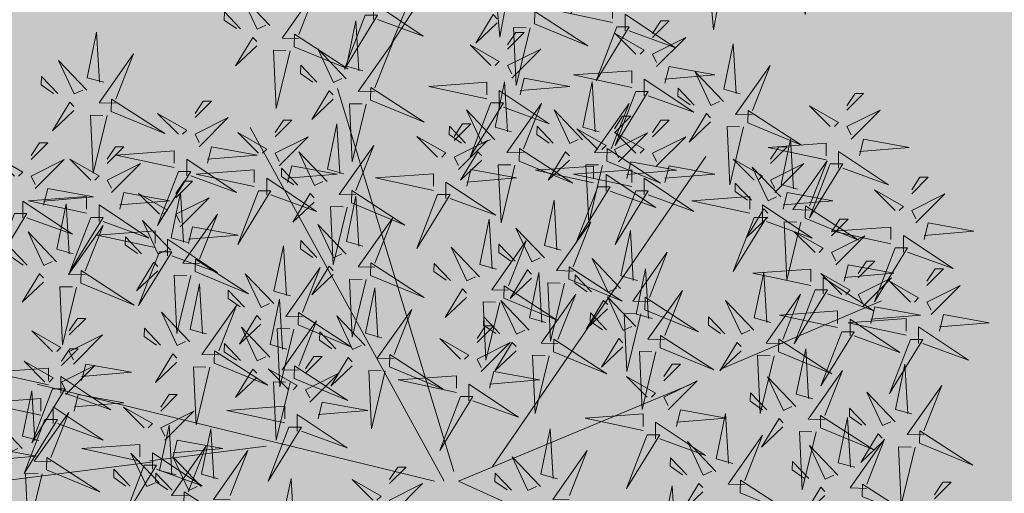
# Model space of a CAD drawing. Units: inches. Extents: x 1704 to 6393, y -157 to 1172.
# Tile 109 of 122: x 2688 to 2716, y 989 to 1003. Entities that reach past the tile are written whole.
import ezdxf

# ---------------------------------------------------------------- set-up
doc = ezdxf.new("R2010")
doc.units = ezdxf.units.IN
doc.header["$MEASUREMENT"] = 0
doc.layers.add('A-ANNO-DIMS', color=7, linetype='Continuous', lineweight=13)
doc.layers.add('L-shrub', color=74, linetype='Continuous', lineweight=18)
doc.layers.add('L-HRDS-PATT', color=9, linetype='Continuous', lineweight=13, true_color=0xc5c1ba)
doc.styles.get("Standard").update_dxf_attribs({"font": 'arial.ttf'})
doc.dimstyles.get("Standard").update_dxf_attribs({"dimtxt": 6, "dimasz": 2, "dimexe": 0.18, "dimexo": 0.0625, "dimgap": 0.09, "dimtad": 0, "dimtih": 1, "dimtoh": 1, "dimdec": 1, "dimzin": 0, "dimdsep": 46, "dimlunit": 3, "dimtxsty": 'Standard', "dimblk": 'ARCHTICK', "dimcen": 0.09, "dimadec": 0, "dimazin": 0, "dimtfac": 1, "dimtdec": 1, "dimtofl": 0, "dimtmove": 0, "dimatfit": 3, "dimfxl": 1, "dimtolj": 1, "dimtzin": 0, "dimarcsym": 0})

# ---------------------------------------------------------------- blocks, each defined once
blk = doc.blocks.new('shrub3')
for p, q in [((-68.47, 143.52), (-106.19, 232.32)), ((-5.99, -2.5), (58.67, 140.12)), ((-14.08, 16.34), (-186.51, 134.74)), ((-5.99, -2.5), (-59.88, 126.66)), ((-11.38, -5.19), (-224.23, -69.78)), ((-5.99, -10.57), (-202.68, -118.21)), ((-5.99, -15.96), (-59.88, -236.62)), ((-17.27, -174.02), (-25.36, -109.43)), ((-16.77, -172.03), (-3.3, -276.98))]:
    blk.add_line(p, q)
for points in [[(29.32, 268.76), (20.08, 271.07), (24.7, 296.43), (27.01, 268.76)], [(72.58, 270.39), (84.86, 300.11), (65.67, 270.57), (72.58, 270.39)], [(-89.4, 264.53), (-98.64, 266.83), (-94.02, 292.2), (-91.71, 264.53)], [(-140.28, 256.06), (-149.52, 258.36), (-144.9, 283.73), (-142.59, 256.06)], [(-82.48, 253), (-91.71, 253), (-73.24, 280.67), (-82.48, 255.31)], [(-27.06, 253.45), (-14.78, 283.17), (-33.97, 253.63), (-27.06, 253.45)], [(-98.64, 259.92), (-114.8, 276.06), (-105.56, 257.61), (-100.94, 259.92)], [(-133.36, 244.53), (-142.59, 244.53), (-124.12, 272.2), (-133.36, 246.84)], [(3.92, 261.85), (-5.31, 271.07), (-5.31, 266.46), (1.62, 261.85)], [(-149.52, 251.45), (-165.68, 267.59), (-156.44, 249.14), (-151.83, 251.45)], [(-114.8, 257.61), (-124.03, 266.83), (-124.03, 262.22), (-117.11, 257.61)], [(-31.61, 255.88), (-31.84, 246.65), (-59.04, 265.8), (-33.91, 255.94)], [(-165.68, 249.14), (-174.91, 258.36), (-174.91, 253.75), (-167.99, 249.14)], [(-105.56, 248.39), (-117.11, 236.86), (-107.87, 253), (-105.56, 250.69)], [(-93.64, 226.42), (-102.88, 228.72), (-98.26, 254.08), (-95.95, 226.42)], [(-84.78, 248.39), (-54.77, 236.86), (-84.78, 255.31), (-84.78, 248.39)], [(-186.92, 220.06), (-196.16, 222.37), (-191.54, 247.73), (-189.23, 220.06)], [(-135.66, 239.92), (-105.65, 228.39), (-135.66, 246.84), (-135.66, 239.92)], [(-43.31, 249.24), (-45.84, 240.07), (-71.08, 245.32), (-43.37, 246.93)], [(-24.81, 251.09), (7.29, 243.36), (-25.04, 241.86), (-24.87, 248.78)], [(2.62, 221.69), (14.9, 251.41), (-4.29, 221.87), (2.62, 221.69)], [(-156.44, 239.92), (-167.99, 228.39), (-158.75, 244.53), (-156.44, 242.22)], [(-87.09, 246.08), (-94.02, 213.8), (-96.33, 246.08), (-89.4, 246.08)], [(-86.72, 214.89), (-95.95, 214.89), (-77.48, 242.56), (-86.72, 217.19)], [(-180, 208.53), (-189.23, 208.53), (-170.76, 236.2), (-180, 210.84)], [(-137.97, 237.61), (-144.9, 205.33), (-147.21, 237.61), (-140.28, 237.61)], [(-116.96, 211.59), (-126.2, 213.9), (-121.58, 239.26), (-119.27, 211.59)], [(-102.88, 221.8), (-119.04, 237.94), (-109.8, 219.5), (-105.18, 221.8)], [(-38.93, 239.9), (-55.47, 224.14), (-36.8, 232.91), (-38.99, 237.59)], [(-196.16, 215.45), (-212.32, 231.59), (-203.08, 213.15), (-198.47, 215.45)], [(-27.58, 232.68), (-16.34, 220.86), (-32.24, 230.49), (-29.88, 232.74)], [(-1.93, 224.12), (-2.16, 214.89), (-29.36, 234.04), (-4.23, 224.17)], [(-119.04, 219.5), (-128.27, 228.72), (-128.27, 224.11), (-121.35, 219.5)], [(-110.04, 200.06), (-119.27, 200.06), (-100.8, 227.73), (-110.04, 202.37)], [(-35.54, 198.4), (-23.26, 228.12), (-42.45, 198.58), (-35.54, 198.4)], [(-212.32, 213.15), (-221.55, 222.37), (-221.55, 217.76), (-214.63, 213.15)], [(-152.14, 189.93), (-139.86, 219.65), (-159.05, 190.11), (-152.14, 189.93)], [(-126.2, 206.98), (-142.36, 223.12), (-133.12, 204.68), (-128.5, 206.98)], [(-37.03, 223.68), (-46.48, 214.68), (-41.87, 214.57), (-37.09, 221.37)], [(-142.36, 204.68), (-151.59, 213.9), (-151.59, 209.29), (-144.67, 204.68)], [(-109.8, 210.27), (-121.35, 198.75), (-112.11, 214.89), (-109.8, 212.58)], [(-89.02, 210.27), (-59.01, 198.75), (-89.02, 217.19), (-89.02, 210.27)], [(-13.63, 217.48), (-16.16, 208.31), (-41.4, 213.56), (-13.69, 215.17)], [(-203.08, 203.92), (-214.63, 192.39), (-205.39, 208.53), (-203.08, 206.23)], [(-182.31, 203.92), (-152.29, 192.39), (-182.31, 210.84), (-182.31, 203.92)], [(-91.33, 207.97), (-98.26, 175.69), (-100.57, 207.97), (-93.64, 207.97)], [(-40.09, 200.83), (-40.32, 191.59), (-67.52, 210.75), (-42.39, 200.88)], [(-9.25, 208.13), (-25.79, 192.38), (-7.12, 201.15), (-9.31, 205.83)], [(-157.24, 177.72), (-166.48, 180.02), (-161.86, 205.38), (-159.55, 177.72)], [(-112.34, 195.45), (-82.33, 183.92), (-112.34, 202.37), (-112.34, 195.45)], [(-77.94, 175.11), (-65.66, 204.83), (-84.85, 175.28), (-77.94, 175.11)], [(-184.61, 201.62), (-191.54, 169.34), (-193.85, 201.62), (-186.92, 201.62)], [(-156.69, 192.36), (-156.92, 183.12), (-184.12, 202.28), (-159, 192.41)], [(-133.12, 195.45), (-144.67, 183.92), (-135.43, 200.06), (-133.12, 197.76)], [(2.1, 200.92), (13.34, 189.09), (-2.56, 198.73), (-0.2, 200.98)], [(-150.32, 166.19), (-159.55, 166.19), (-141.08, 193.86), (-150.32, 168.49)], [(-114.65, 193.15), (-121.58, 160.87), (-123.89, 193.15), (-116.96, 193.15)], [(-51.79, 194.19), (-54.32, 185.02), (-79.56, 190.27), (-51.85, 191.88)], [(-33.29, 196.04), (-1.19, 188.31), (-33.52, 186.81), (-33.35, 193.73)], [(-7.35, 191.92), (-16.8, 182.92), (-12.19, 182.81), (-7.41, 189.61)], [(-205.14, 158.17), (-192.86, 187.89), (-212.05, 158.35), (-205.14, 158.17)], [(-166.48, 173.1), (-182.64, 189.24), (-173.4, 170.8), (-168.79, 173.1)], [(-149.89, 187.57), (-117.79, 179.84), (-150.12, 178.34), (-149.95, 185.26)], [(-82.49, 177.53), (-82.72, 168.3), (-109.92, 187.46), (-84.79, 177.59)], [(-168.39, 185.72), (-170.92, 176.55), (-196.16, 181.8), (-168.45, 183.41)], [(-47.41, 184.84), (-63.95, 169.09), (-45.28, 177.86), (-47.47, 182.54)], [(0.5, 153.94), (12.78, 183.65), (-6.41, 154.11), (0.5, 153.94)], [(-182.64, 170.8), (-191.87, 180.02), (-191.87, 175.41), (-184.95, 170.8)], [(-164.01, 176.37), (-180.55, 160.62), (-161.88, 169.39), (-164.07, 174.07)], [(-36.06, 177.63), (-24.82, 165.8), (-40.72, 175.44), (-38.36, 177.69)], [(-209.69, 160.6), (-209.92, 151.36), (-237.12, 170.52), (-212, 160.65)], [(-94.19, 170.9), (-96.72, 161.73), (-121.96, 166.98), (-94.25, 168.59)], [(-75.69, 172.75), (-43.59, 165.01), (-75.92, 163.51), (-75.75, 170.44)], [(-173.4, 161.57), (-184.95, 150.05), (-175.71, 166.19), (-173.4, 163.88)], [(-152.66, 169.16), (-141.42, 157.33), (-157.33, 166.97), (-154.96, 169.22)], [(-152.62, 161.57), (-122.61, 150.05), (-152.62, 168.49), (-152.62, 161.57)], [(-45.51, 168.63), (-54.96, 159.63), (-50.35, 159.51), (-45.57, 166.32)], [(-4.05, 156.36), (-4.28, 147.13), (-31.48, 166.28), (-6.35, 156.42)], [(-162.11, 160.16), (-171.56, 151.16), (-166.95, 151.04), (-162.17, 157.85)], [(-154.93, 159.27), (-161.86, 126.99), (-164.17, 159.27), (-157.24, 159.27)], [(-89.81, 161.55), (-106.35, 145.8), (-87.68, 154.57), (-89.87, 159.24)], [(-221.39, 153.96), (-223.93, 144.79), (-249.17, 150.04), (-221.45, 151.65)], [(-202.89, 155.81), (-170.79, 148.07), (-203.12, 146.57), (-202.95, 153.5)], [(-78.46, 154.34), (-67.22, 142.51), (-83.13, 152.15), (-80.76, 154.4)], [(-15.75, 149.73), (-18.28, 140.55), (-43.52, 145.8), (-15.81, 147.42)], [(-217.01, 144.61), (-233.55, 128.86), (-214.88, 137.63), (-217.07, 142.31)], [(-87.91, 145.34), (-97.36, 136.34), (-92.75, 136.22), (-87.97, 143.03)], [(-36.4, 118.43), (-45.64, 120.73), (-41.02, 146.1), (-38.71, 118.43)], [(-227.2, 112.08), (-236.44, 114.38), (-231.82, 139.75), (-229.51, 112.08)], [(-205.66, 137.4), (-194.42, 125.57), (-210.33, 135.21), (-207.96, 137.46)], [(-172.08, 112.08), (-181.32, 114.38), (-176.7, 139.75), (-174.39, 112.08)], [(-80.06, 109.47), (-67.78, 139.19), (-86.97, 109.65), (-80.06, 109.47)], [(-11.37, 140.38), (-27.91, 124.63), (-9.24, 133.4), (-11.43, 138.07)], [(-29.48, 106.9), (-38.71, 106.9), (-20.24, 134.57), (-29.48, 109.2)], [(-0.02, 133.17), (11.22, 121.34), (-4.68, 130.97), (-2.32, 133.22)], [(-220.28, 100.55), (-229.51, 100.55), (-211.04, 128.22), (-220.28, 102.85)], [(-215.11, 128.4), (-224.56, 119.4), (-219.95, 119.28), (-215.17, 126.09)], [(-165.16, 100.55), (-174.39, 100.55), (-155.92, 128.22), (-165.16, 102.85)], [(-101.26, 101), (-88.98, 130.72), (-108.17, 101.18), (-101.26, 101)], [(-45.64, 113.82), (-61.8, 129.96), (-52.56, 111.51), (-47.94, 113.82)], [(-236.44, 107.46), (-252.6, 123.6), (-243.36, 105.16), (-238.75, 107.46)], [(-181.32, 107.46), (-197.48, 123.6), (-188.24, 105.16), (-183.63, 107.46)], [(-84.61, 111.9), (-84.84, 102.66), (-112.04, 121.82), (-86.91, 111.95)], [(-61.8, 111.51), (-71.03, 120.73), (-71.03, 116.12), (-64.1, 111.51)], [(-9.47, 124.17), (-18.92, 115.16), (-14.31, 115.05), (-9.53, 121.86)], [(-256.32, 89.96), (-265.55, 89.96), (-247.08, 117.63), (-256.32, 92.27)], [(-174.2, 90.9), (-183.44, 93.21), (-178.82, 118.57), (-176.51, 90.9)], [(24.53, 120.08), (22, 110.91), (-3.24, 116.16), (24.47, 117.77)], [(-252.6, 105.16), (-261.83, 114.38), (-261.83, 109.77), (-254.91, 105.16)], [(-197.48, 105.16), (-206.71, 114.38), (-206.71, 109.77), (-199.79, 105.16)], [(-183.94, 79.83), (-171.66, 109.54), (-190.85, 80), (-183.94, 79.83)], [(-105.81, 103.43), (-106.04, 94.19), (-133.24, 113.35), (-108.11, 103.48)], [(-167.28, 79.37), (-176.51, 79.37), (-158.04, 107.04), (-167.28, 81.68)], [(-96.31, 105.26), (-98.84, 96.09), (-124.08, 101.34), (-96.37, 102.95)], [(-77.81, 107.11), (-45.71, 99.37), (-78.04, 97.87), (-77.87, 104.8)], [(-52.56, 102.29), (-64.1, 90.76), (-54.87, 106.9), (-52.56, 104.59)], [(-31.78, 102.29), (-1.77, 90.76), (-31.78, 109.2), (-31.78, 102.29)], [(-243.36, 95.94), (-254.91, 84.41), (-245.67, 100.55), (-243.36, 98.24)], [(-222.59, 95.94), (-192.57, 84.41), (-222.59, 102.85), (-222.59, 95.94)], [(-188.24, 95.94), (-199.79, 84.41), (-190.55, 100.55), (-188.24, 98.24)], [(-183.44, 86.29), (-199.6, 102.43), (-190.36, 83.98), (-185.75, 86.29)], [(-167.46, 95.94), (-137.45, 84.41), (-167.46, 102.85), (-167.46, 95.94)], [(-99.01, 98.64), (-66.91, 90.91), (-99.24, 89.41), (-99.07, 96.33)], [(-34.09, 99.98), (-41.02, 67.7), (-43.33, 99.98), (-36.4, 99.98)], [(-224.89, 93.63), (-231.82, 61.35), (-234.13, 93.63), (-227.2, 93.63)], [(-199.6, 83.98), (-208.83, 93.21), (-208.83, 88.6), (-201.91, 83.98)], [(-169.77, 93.63), (-176.7, 61.35), (-179.01, 93.63), (-172.08, 93.63)], [(-117.51, 96.79), (-120.04, 87.62), (-145.28, 92.87), (-117.57, 94.48)], [(-91.93, 95.91), (-108.47, 80.16), (-89.8, 88.93), (-91.99, 93.61)], [(-258.63, 85.35), (-228.61, 73.82), (-258.63, 92.27), (-258.63, 85.35)], [(-188.49, 82.25), (-188.72, 73.02), (-215.92, 92.18), (-190.8, 82.31)], [(-118.22, 58.65), (-105.94, 88.37), (-125.13, 58.83), (-118.22, 58.65)], [(-80.58, 88.7), (-69.34, 76.87), (-85.25, 86.51), (-82.88, 88.76)], [(-260.93, 83.04), (-267.86, 50.76), (-270.17, 83.04), (-263.24, 83.04)], [(-113.13, 87.44), (-129.67, 71.69), (-111, 80.46), (-113.19, 85.14)], [(-190.36, 74.76), (-201.91, 63.23), (-192.67, 79.37), (-190.36, 77.07)], [(-181.69, 77.46), (-149.59, 69.73), (-181.92, 68.23), (-181.75, 75.15)], [(-169.58, 74.76), (-139.57, 63.23), (-169.58, 81.68), (-169.58, 74.76)], [(-101.78, 80.23), (-90.54, 68.4), (-106.45, 78.04), (-104.08, 80.29)], [(-90.03, 79.7), (-99.48, 70.7), (-94.87, 70.58), (-90.09, 77.39)], [(-77.94, 50.18), (-65.66, 79.9), (-84.85, 50.36), (-77.94, 50.18)], [(-200.19, 75.62), (-202.73, 66.44), (-227.97, 71.69), (-200.25, 73.31)], [(-171.89, 72.46), (-178.82, 40.17), (-181.13, 72.46), (-174.2, 72.46)], [(-111.23, 71.23), (-120.68, 62.23), (-116.07, 62.11), (-111.29, 68.92)], [(-260.26, 39.6), (-247.98, 69.31), (-267.17, 39.77), (-260.26, 39.6)], [(-195.81, 66.27), (-212.35, 50.52), (-193.68, 59.29), (-195.87, 63.96)], [(-122.77, 61.08), (-123, 51.85), (-150.2, 71), (-125.08, 61.14)], [(4.43, 58.96), (4.2, 49.73), (-23, 68.88), (2.13, 59.02)], [(-183.94, 31.13), (-171.66, 60.84), (-190.85, 31.3), (-183.94, 31.13)], [(-82.49, 52.61), (-82.72, 43.38), (-109.92, 62.53), (-84.79, 52.67)], [(-220.84, 31.61), (-230.08, 33.92), (-225.46, 59.28), (-223.15, 31.61)], [(-184.46, 59.06), (-173.22, 47.23), (-189.13, 56.86), (-186.76, 59.12)], [(-115.97, 56.29), (-83.87, 48.56), (-116.2, 47.06), (-116.03, 53.98)], [(-193.91, 50.06), (-203.36, 41.06), (-198.75, 40.94), (-193.97, 47.75)], [(-134.47, 54.44), (-137, 45.27), (-162.24, 50.52), (-134.53, 52.13)], [(-107.62, 22.66), (-95.34, 52.37), (-114.53, 22.83), (-107.62, 22.66)], [(-7.27, 52.33), (-9.8, 43.15), (-35.04, 48.4), (-7.33, 50.02)], [(-213.92, 20.09), (-223.15, 20.09), (-204.68, 47.76), (-213.92, 22.39)], [(-130.09, 45.1), (-146.63, 29.34), (-127.96, 38.11), (-130.15, 42.79)], [(-94.19, 45.97), (-96.72, 36.8), (-121.96, 42.05), (-94.25, 43.67)], [(-75.69, 47.82), (-43.59, 40.09), (-75.92, 38.59), (-75.75, 45.51)], [(-230.08, 27), (-246.24, 43.14), (-237, 24.7), (-232.39, 27)], [(-188.49, 33.55), (-188.72, 24.32), (-215.92, 43.48), (-190.8, 33.61)], [(-57.6, 14.68), (-66.84, 16.98), (-62.22, 42.34), (-59.91, 14.68)], [(-2.89, 42.98), (-19.43, 27.23), (-0.76, 36), (-2.95, 40.67)], [(-258.01, 37.23), (-225.91, 29.5), (-258.24, 28), (-258.07, 34.92)], [(-246.24, 24.7), (-255.47, 33.92), (-255.47, 29.31), (-248.55, 24.7)], [(-112.17, 25.08), (-112.4, 15.85), (-139.6, 35.01), (-114.47, 25.14)], [(-118.74, 37.88), (-107.5, 26.06), (-123.41, 35.69), (-121.04, 37.94)], [(-89.81, 36.63), (-106.35, 20.87), (-87.68, 29.64), (-89.87, 34.32)], [(-181.69, 28.76), (-149.59, 21.03), (-181.92, 19.53), (-181.75, 26.45)], [(-169.96, 1.97), (-179.2, 4.28), (-174.58, 29.64), (-172.27, 1.97)], [(-128.19, 28.88), (-137.64, 19.88), (-133.03, 19.77), (-128.25, 26.57)], [(-78.46, 29.41), (-67.22, 17.59), (-83.13, 27.22), (-80.76, 29.47)], [(-50.68, 3.15), (-59.91, 3.15), (-41.44, 30.82), (-50.68, 5.45)], [(-200.19, 26.92), (-202.73, 17.74), (-227.97, 22.99), (-200.25, 24.61)], [(-216.23, 15.47), (-186.21, 3.95), (-216.23, 22.39), (-216.23, 15.47)], [(-66.84, 10.06), (-83, 26.2), (-73.76, 7.76), (-69.14, 10.06)], [(-0.99, 26.77), (-10.44, 17.76), (-5.83, 17.65), (-1.05, 24.46)], [(-260.78, 18.83), (-249.54, 7), (-265.45, 16.63), (-263.08, 18.88)], [(-237, 15.47), (-248.55, 3.95), (-239.31, 20.09), (-237, 17.78)], [(-195.81, 17.57), (-212.35, 1.82), (-193.68, 10.59), (-195.87, 15.26)], [(-163.04, -9.56), (-172.27, -9.56), (-153.8, 18.11), (-163.04, -7.25)], [(-123.87, 18.45), (-126.4, 9.27), (-151.64, 14.52), (-123.93, 16.14)], [(-105.37, 20.29), (-73.27, 12.56), (-105.6, 11.06), (-105.43, 17.99)], [(-87.91, 20.41), (-97.36, 11.41), (-92.75, 11.3), (-87.97, 18.11)], [(-83, 7.76), (-92.23, 16.98), (-92.23, 12.37), (-85.3, 7.76)], [(-218.53, 13.17), (-225.46, -19.11), (-227.77, 13.17), (-220.84, 13.17)], [(-179.2, -2.64), (-195.36, 13.5), (-186.12, -4.95), (-181.51, -2.64)], [(-184.46, 10.36), (-173.22, -1.47), (-189.13, 8.16), (-186.76, 10.41)], [(-119.49, 9.1), (-136.03, -6.65), (-117.36, 2.12), (-119.55, 6.79)], [(-195.36, -4.95), (-204.59, 4.28), (-204.59, -0.33), (-197.67, -4.95)], [(-193.91, 1.36), (-203.36, -7.64), (-198.75, -7.76), (-193.97, -0.95)], [(-108.14, 1.89), (-96.9, -9.94), (-112.81, -0.3), (-110.44, 1.95)], [(-73.76, -1.46), (-85.3, -12.99), (-76.07, 3.15), (-73.76, 0.84)], [(-52.98, -1.46), (-22.97, -12.99), (-52.98, 5.45), (-52.98, -1.46)], [(-55.29, -3.77), (-62.22, -36.05), (-64.53, -3.77), (-57.6, -3.77)], [(-186.12, -14.17), (-197.67, -25.7), (-188.43, -9.56), (-186.12, -11.86)], [(-165.34, -14.17), (-135.33, -25.7), (-165.34, -7.25), (-165.34, -14.17)], [(-117.59, -7.11), (-127.04, -16.11), (-122.43, -16.23), (-117.65, -9.42)], [(-69.46, -40.86), (-57.18, -11.15), (-76.37, -40.69), (-69.46, -40.86)], [(-217.86, -51.45), (-205.58, -21.74), (-224.77, -51.28), (-217.86, -51.45)], [(-167.65, -16.47), (-174.58, -48.76), (-176.89, -16.47), (-169.96, -16.47)], [(-120.34, -51.45), (-108.06, -21.74), (-127.25, -51.28), (-120.34, -51.45)], [(-262.68, -49.79), (-271.91, -49.79), (-253.44, -22.12), (-262.68, -47.48)], [(11.6, -38.64), (-4.56, -22.5), (4.68, -40.94), (9.3, -38.64)], [(-160.62, -62.04), (-148.34, -32.32), (-167.53, -61.86), (-160.62, -62.04)], [(-74.01, -38.44), (-74.24, -47.67), (-101.44, -28.52), (-76.31, -38.38)], [(-4.56, -40.94), (-13.79, -31.72), (-13.79, -36.33), (-6.86, -40.94)], [(-222.41, -49.03), (-222.64, -58.26), (-249.84, -39.1), (-224.72, -48.97)], [(-124.89, -49.03), (-125.12, -58.26), (-152.32, -39.1), (-127.2, -48.97)], [(-67.21, -43.23), (-35.11, -50.96), (-67.44, -52.46), (-67.27, -45.54)], [(-264.99, -54.4), (-234.97, -65.93), (-264.99, -47.48), (-264.99, -54.4)], [(-85.71, -45.07), (-88.24, -54.25), (-113.48, -49), (-85.77, -47.38)], [(4.68, -50.16), (-6.86, -61.69), (2.37, -45.55), (4.68, -47.86)], [(-215.61, -53.82), (-183.51, -61.55), (-215.84, -63.05), (-215.67, -56.12)], [(-165.17, -59.61), (-165.4, -68.85), (-192.6, -49.69), (-167.48, -59.56)], [(-118.09, -53.82), (-85.99, -61.55), (-118.32, -63.05), (-118.15, -56.12)], [(-81.33, -54.42), (-97.87, -70.17), (-79.2, -61.4), (-81.39, -56.73)], [(-40.64, -80.61), (-49.88, -78.3), (-45.26, -52.94), (-42.95, -80.61)], [(-234.11, -55.66), (-236.65, -64.84), (-261.89, -59.59), (-234.17, -57.97)], [(-136.59, -55.66), (-139.12, -64.84), (-164.36, -59.59), (-136.65, -57.97)], [(-247.54, -93.8), (-235.26, -64.08), (-254.45, -93.62), (-247.54, -93.8)], [(-229.73, -65.01), (-246.27, -80.76), (-227.6, -71.99), (-229.79, -67.32)], [(-158.37, -64.4), (-126.27, -72.13), (-158.6, -73.63), (-158.43, -66.71)], [(-132.21, -65.01), (-148.75, -80.76), (-130.08, -71.99), (-132.27, -67.32)], [(-92.78, -91.68), (-80.5, -61.97), (-99.69, -91.51), (-92.78, -91.68)], [(-69.98, -61.63), (-58.74, -73.46), (-74.65, -63.83), (-72.28, -61.58)], [(-63.1, -93.8), (-50.82, -64.08), (-70.01, -93.62), (-63.1, -93.8)], [(-33.72, -92.14), (-42.95, -92.14), (-24.48, -64.47), (-33.72, -89.83)], [(-176.87, -66.25), (-179.4, -75.42), (-204.64, -70.17), (-176.93, -68.56)], [(-172.08, -97.55), (-181.32, -95.24), (-176.7, -69.88), (-174.39, -97.55)], [(-79.43, -70.63), (-88.88, -79.64), (-84.27, -79.75), (-79.49, -72.94)], [(-49.88, -85.22), (-66.04, -69.08), (-56.8, -87.52), (-52.18, -85.22)], [(-218.38, -72.22), (-207.14, -84.05), (-223.05, -74.41), (-220.68, -72.16)], [(-172.49, -75.6), (-189.03, -91.35), (-170.36, -82.58), (-172.55, -77.9)], [(-120.86, -72.22), (-109.62, -84.05), (-125.53, -74.41), (-123.16, -72.16)], [(-252.09, -91.37), (-252.32, -100.61), (-279.52, -81.45), (-254.4, -91.32)], [(-227.83, -81.22), (-237.28, -90.22), (-232.67, -90.34), (-227.89, -83.53)], [(-165.16, -109.08), (-174.39, -109.08), (-155.92, -81.41), (-165.16, -106.77)], [(-130.31, -81.22), (-139.76, -90.22), (-135.15, -90.34), (-130.37, -83.53)], [(-97.33, -89.26), (-97.56, -98.49), (-124.76, -79.33), (-99.63, -89.2)], [(-67.65, -91.37), (-67.88, -100.61), (-95.08, -81.45), (-69.95, -91.32)], [(-66.04, -87.52), (-75.27, -78.3), (-75.27, -82.91), (-68.34, -87.52)], [(-181.32, -102.16), (-197.48, -86.02), (-188.24, -104.46), (-183.63, -102.16)], [(-161.14, -82.81), (-149.9, -94.64), (-165.81, -85), (-163.44, -82.75)], [(-170.59, -91.81), (-180.04, -100.81), (-175.43, -100.93), (-170.65, -94.12)], [(-56.8, -96.75), (-68.34, -108.28), (-59.11, -92.14), (-56.8, -94.44)], [(-36.02, -96.75), (-6.01, -108.28), (-36.02, -89.83), (-36.02, -96.75)], [(20.29, -91.66), (17.76, -100.83), (-7.48, -95.58), (20.23, -93.97)], [(-245.29, -96.16), (-213.19, -103.89), (-245.52, -105.4), (-245.35, -98.47)], [(-197.48, -104.46), (-206.71, -95.24), (-206.71, -99.85), (-199.79, -104.46)], [(-109.03, -95.89), (-111.56, -105.07), (-136.8, -99.82), (-109.09, -98.2)], [(-79.35, -98.01), (-81.88, -107.18), (-107.12, -101.93), (-79.41, -100.32)], [(-90.53, -94.05), (-58.43, -101.78), (-90.76, -103.28), (-90.59, -96.35)], [(-60.85, -96.16), (-28.75, -103.89), (-61.08, -105.4), (-60.91, -98.47)], [(-38.33, -99.05), (-45.26, -131.33), (-47.57, -99.05), (-40.64, -99.05)], [(-259.41, -107.36), (-275.95, -123.11), (-257.28, -114.34), (-259.47, -109.66)], [(-188.24, -113.69), (-199.79, -125.22), (-190.55, -109.08), (-188.24, -111.38)], [(-167.46, -113.69), (-137.45, -125.22), (-167.46, -106.77), (-167.46, -113.69)], [(-104.65, -105.24), (-121.19, -120.99), (-102.52, -112.22), (-104.71, -107.55)], [(-74.97, -107.36), (-91.51, -123.11), (-72.84, -114.34), (-75.03, -109.66)], [(-71.58, -138.26), (-59.3, -108.55), (-78.49, -138.09), (-71.58, -138.26)], [(-248.06, -114.57), (-236.82, -126.4), (-252.73, -116.76), (-250.36, -114.51)], [(-182.68, -142.01), (-191.92, -139.71), (-187.3, -114.34), (-184.99, -142.01)], [(-93.3, -112.45), (-82.06, -124.28), (-97.97, -114.64), (-95.6, -112.39)], [(-63.62, -114.57), (-52.38, -126.4), (-68.29, -116.76), (-65.92, -114.51)], [(-169.77, -115.99), (-176.7, -148.27), (-179.01, -115.99), (-172.08, -115.99)], [(-122.46, -148.85), (-110.18, -119.14), (-129.37, -148.68), (-122.46, -148.85)], [(4.43, -129.49), (4.2, -138.72), (-23, -119.56), (2.13, -129.43)], [(-257.51, -123.57), (-266.96, -132.57), (-262.35, -132.69), (-257.57, -125.88)], [(-138.16, -152.6), (-147.4, -150.29), (-142.78, -124.93), (-140.47, -152.6)], [(-102.75, -121.45), (-112.2, -130.45), (-107.59, -130.57), (-102.81, -123.76)], [(-73.07, -123.57), (-82.52, -132.57), (-77.91, -132.69), (-73.13, -125.88)], [(6.86, -155.2), (19.14, -125.49), (-0.05, -155.03), (6.86, -155.2)], [(-191.92, -146.62), (-208.08, -130.48), (-198.84, -148.93), (-194.23, -146.62)], [(-175.76, -153.54), (-184.99, -153.54), (-166.52, -125.87), (-175.76, -151.23)], [(-76.13, -135.84), (-76.36, -145.07), (-103.56, -125.92), (-78.43, -135.78)], [(-127.01, -146.43), (-127.24, -155.66), (-154.44, -136.5), (-129.32, -146.37)], [(-131.24, -164.13), (-140.47, -164.13), (-122, -136.46), (-131.24, -161.82)], [(-7.27, -136.12), (-9.8, -145.3), (-35.04, -140.05), (-7.33, -138.43)], [(-19.44, -161.07), (-28.68, -158.76), (-24.06, -133.4), (-21.75, -161.07)], [(-208.08, -148.93), (-217.31, -139.71), (-217.31, -144.32), (-210.39, -148.93)], [(-147.4, -157.21), (-163.56, -141.07), (-154.32, -159.52), (-149.71, -157.21)], [(-69.33, -140.63), (-37.23, -148.36), (-69.56, -149.86), (-69.39, -142.94)], [(-87.83, -142.48), (-90.36, -151.65), (-115.6, -146.4), (-87.89, -144.78)], [(2.31, -152.78), (2.08, -162.01), (-25.12, -142.86), (0.01, -152.72)], [(-12.52, -172.6), (-21.75, -172.6), (-3.28, -144.93), (-12.52, -170.29)], [(-2.89, -145.47), (-19.43, -161.22), (-0.76, -152.45), (-2.95, -147.78)], [(-178.06, -158.15), (-148.05, -169.68), (-178.06, -151.23), (-178.06, -158.15)], [(-163.56, -159.52), (-172.79, -150.29), (-172.79, -154.9), (-165.87, -159.52)], [(-138.71, -153.06), (-141.24, -162.24), (-166.48, -156.99), (-138.77, -155.37)], [(-120.21, -151.22), (-88.11, -158.95), (-120.44, -160.45), (-120.27, -153.52)], [(-83.45, -151.82), (-99.99, -167.57), (-81.32, -158.8), (-83.51, -154.13)], [(-28.68, -165.68), (-44.84, -149.54), (-35.6, -167.99), (-30.98, -165.68)], [(-198.84, -158.15), (-210.39, -169.68), (-201.15, -153.54), (-198.84, -155.85)], [(-180.37, -160.46), (-187.3, -192.74), (-189.61, -160.46), (-182.68, -160.46)], [(-157.24, -190.71), (-166.48, -188.41), (-161.86, -163.04), (-159.55, -190.71)], [(-134.33, -162.41), (-150.87, -178.16), (-132.2, -169.39), (-134.39, -164.72)], [(-133.54, -168.74), (-103.53, -180.27), (-133.54, -161.82), (-133.54, -168.74)], [(-72.1, -159.03), (-60.86, -170.86), (-76.77, -161.23), (-74.4, -158.98)], [(-44.84, -167.99), (-54.07, -158.76), (-54.07, -163.37), (-47.14, -167.99)], [(-9.39, -159.41), (-11.92, -168.59), (-37.16, -163.34), (-9.45, -161.72)], [(-0.99, -161.68), (-10.44, -170.68), (-5.83, -170.8), (-1.05, -163.99)], [(-211.5, -195.43), (-199.22, -165.72), (-218.41, -195.26), (-211.5, -195.43)], [(-154.32, -168.74), (-165.87, -180.27), (-156.63, -164.13), (-154.32, -166.43)], [(-81.55, -168.04), (-91, -177.04), (-86.39, -177.15), (-81.61, -170.34)], [(-5.01, -168.76), (-21.55, -184.51), (-2.88, -175.74), (-5.07, -171.07)], [(-150.32, -202.24), (-159.55, -202.24), (-141.08, -174.57), (-150.32, -199.93)], [(-135.85, -171.04), (-142.78, -203.33), (-145.09, -171.04), (-138.16, -171.04)], [(-122.98, -169.62), (-111.74, -181.45), (-127.65, -171.81), (-125.28, -169.56)], [(-35.6, -177.21), (-47.14, -188.74), (-37.91, -172.6), (-35.6, -174.9)], [(-14.82, -177.21), (15.19, -188.74), (-14.82, -170.29), (-14.82, -177.21)], [(-166.48, -195.32), (-182.64, -179.18), (-173.4, -197.63), (-168.79, -195.32)], [(-132.43, -178.62), (-141.88, -187.62), (-137.27, -187.74), (-132.49, -180.93)], [(-17.13, -179.51), (-24.06, -211.79), (-26.37, -179.51), (-19.44, -179.51)], [(-216.05, -193.01), (-216.28, -202.24), (-243.48, -183.09), (-218.36, -192.95)], [(-116.1, -212.37), (-103.82, -182.66), (-123.01, -212.2), (-116.1, -212.37)], [(-61.84, -211.89), (-71.08, -209.58), (-66.46, -184.22), (-64.15, -211.89)], [(-3.11, -184.97), (-12.56, -193.97), (-7.95, -194.09), (-3.17, -187.28)], [(-182.64, -197.63), (-191.87, -188.41), (-191.87, -193.02), (-184.95, -197.63)], [(-44.88, -216.12), (-54.12, -213.81), (-49.5, -188.45), (-47.19, -216.12)], [(-54.92, -223.41), (-64.15, -223.41), (-45.68, -195.75), (-54.92, -221.11)], [(-227.75, -199.64), (-230.29, -208.82), (-255.53, -203.57), (-227.81, -201.95)], [(-209.25, -197.8), (-177.15, -205.53), (-209.48, -207.03), (-209.31, -200.11)], [(-173.4, -206.85), (-184.95, -218.38), (-175.71, -202.24), (-173.4, -204.55)], [(-152.62, -206.85), (-122.61, -218.38), (-152.62, -199.93), (-152.62, -206.85)], [(-120.65, -209.95), (-120.88, -219.18), (-148.08, -200.02), (-122.96, -209.89)], [(-71.08, -216.5), (-87.24, -200.36), (-78, -218.8), (-73.38, -216.5)], [(-37.96, -227.65), (-47.19, -227.65), (-28.72, -199.98), (-37.96, -225.34)], [(-12.22, -231.43), (0.06, -201.71), (-19.13, -231.26), (-12.22, -231.43)], [(-159.36, -233.06), (-168.6, -230.75), (-163.98, -205.39), (-161.67, -233.06)], [(-54.12, -220.73), (-70.28, -204.59), (-61.04, -223.04), (-56.42, -220.73)], [(-223.37, -208.99), (-239.91, -224.74), (-221.24, -215.97), (-223.43, -211.3)], [(-154.93, -209.16), (-161.86, -241.44), (-164.17, -209.16), (-157.24, -209.16)], [(-87.24, -218.8), (-96.47, -209.58), (-96.47, -214.19), (-89.54, -218.8)], [(-212.02, -216.2), (-200.78, -228.03), (-216.69, -218.4), (-214.32, -216.15)], [(-152.44, -244.59), (-161.67, -244.59), (-143.2, -216.92), (-152.44, -242.28)], [(-132.35, -216.58), (-134.88, -225.76), (-160.12, -220.51), (-132.41, -218.89)], [(-113.85, -214.74), (-81.75, -222.47), (-114.08, -223.97), (-113.91, -217.05)], [(-70.28, -223.04), (-79.51, -213.81), (-79.51, -218.43), (-72.58, -223.04)], [(-168.6, -237.67), (-184.76, -221.53), (-175.52, -239.98), (-170.91, -237.67)], [(-78, -228.03), (-89.54, -239.55), (-80.31, -223.41), (-78, -225.72)], [(-57.22, -228.03), (-27.21, -239.55), (-57.22, -221.11), (-57.22, -228.03)], [(-16.77, -229.01), (-17, -238.24), (-44.2, -219.08), (-19.07, -228.95)], [(-221.47, -225.2), (-230.92, -234.21), (-226.31, -234.32), (-221.53, -227.51)], [(-127.97, -225.93), (-144.51, -241.68), (-125.84, -232.91), (-128.03, -228.24)], [(-61.04, -232.26), (-72.58, -243.79), (-63.35, -227.65), (-61.04, -229.95)], [(-40.26, -232.26), (-10.25, -243.79), (-40.26, -225.34), (-40.26, -232.26)], [(-184.76, -239.98), (-193.99, -230.75), (-193.99, -235.37), (-187.07, -239.98)], [(-116.62, -233.14), (-105.38, -244.97), (-121.29, -235.34), (-118.92, -233.09)], [(-59.53, -230.33), (-66.46, -262.61), (-68.77, -230.33), (-61.84, -230.33)], [(-42.57, -234.57), (-49.5, -266.85), (-51.81, -234.57), (-44.88, -234.57)], [(-9.97, -233.79), (22.13, -241.53), (-10.2, -243.03), (-10.03, -236.1)], [(-28.47, -235.64), (-31, -244.81), (-56.24, -239.56), (-28.53, -237.95)], [(-15.2, -264.82), (-24.44, -262.51), (-19.82, -237.15), (-17.51, -264.82)], [(-175.52, -249.2), (-187.07, -260.73), (-177.83, -244.59), (-175.52, -246.89)], [(-154.74, -249.2), (-124.73, -260.73), (-154.74, -242.28), (-154.74, -249.2)], [(-126.07, -242.14), (-135.52, -251.14), (-130.91, -251.26), (-126.13, -244.45)], [(-24.09, -244.99), (-40.63, -260.74), (-21.96, -251.97), (-24.15, -247.3)]]:
    blk.add_lwpolyline(points)
blk = doc.blocks.new('_ArchTick')
at = {"color": 0, "linetype": 'ByBlock', "const_width": 0.15}
blk.add_lwpolyline([(-0.5, -0.5), (0.5, 0.5)], dxfattribs=at)
blk = doc.blocks.new('*D95')
at = {"layer": 'A-ANNO-DIMS', "color": 0, "lineweight": -2, "transparency": 16777216}
for p, q in [((2605.349, 895.275), (2605.349, 1105.287)), ((2723.349, 895.275), (2723.349, 1105.287)), ((2605.349, 1105.107), (2657.907, 1105.107)), ((2723.349, 1105.107), (2670.791, 1105.107))]:
    blk.add_line(p, q, dxfattribs=at)
at = {"layer": 'Defpoints', "color": 0, "lineweight": -3, "transparency": 16777216}
for p in [(2723.349, 1105.107), (2605.349, 895.213), (2723.349, 895.213)]:
    blk.add_point(p, dxfattribs=at)
at = {"layer": 'A-ANNO-DIMS', "color": 0, "lineweight": -2, "transparency": 16777216, "xscale": 2, "yscale": 2, "zscale": 2, "rotation": 180}
blk.add_blockref('_ArchTick', (2605.349, 1105.107), dxfattribs=at)
at = {"layer": 'A-ANNO-DIMS', "color": 0, "lineweight": -2, "transparency": 16777216, "xscale": 2, "yscale": 2, "zscale": 2}
blk.add_blockref('_ArchTick', (2723.349, 1105.107), dxfattribs=at)
at = {"layer": 'A-ANNO-DIMS', "color": 0, "transparency": 16777216, "insert": (2664.349, 1105.107), "char_height": 6, "attachment_point": 5}
blk.add_mtext('\\A1;118', dxfattribs=at)

msp = doc.modelspace()

# ---------------------------------------------------------------- hatches: boundary and pattern name
at = {"layer": 'L-HRDS-PATT', "transparency": 33554661}
h = msp.add_hatch(color=256, dxfattribs=at)
h.dxf.hatch_style = 1
h.paths.add_polyline_path([(2719.349, 1033.213), (2664.349, 1033.213), (2664.349, 895.213), (2719.349, 895.213)])
h.paths.add_polyline_path([(2719.349, 895.213), (2664.349, 895.213), (2605.349, 895.213), (2605.349, 872.213), (2719.349, 872.213)])
h.paths.add_polyline_path([(2719.349, 872.213), (2605.349, 872.213), (2605.349, 854.213), (2601.349, 854.213, -0.121066), (2618.034, 850.113), (2618.05, 850.14), (2619.349, 849.39), (2601.349, 818.213), (2605.349, 818.213), (2605.349, 794.213), (2605.349, 754.213), (2631.349, 754.213), (2631.349, 716.213), (2719.349, 716.213)])

# ---------------------------------------------------------------- block references
at = {"layer": 'L-shrub', "xscale": 0.0510581485411622, "yscale": 0.0510581485411622, "zscale": 0.0510581485411622}
for p, rotation in [((2703.343, 1017.291), 180), ((2701.044, 989.25), 269.9999999999999)]:
    msp.add_blockref('shrub3', p, dxfattribs=dict(at, rotation=rotation))

# ---------------------------------------------------------------- dimensions: what is measured, and where the dimension line sits
at = {"layer": 'A-ANNO-DIMS'}
dim = msp.add_linear_dim(base=(2723.349, 1105.107), p1=(2605.349, 895.213), p2=(2723.349, 895.213), dimstyle='Standard', override={"dimdec": 0, "dimlfac": 1, "dimrnd": 0, "dimzin": 0, "dimdsep": 46, "dimlunit": 2}, dxfattribs=at)
dim.commit()
dim.dimension.update_dxf_attribs({"geometry": '*D95', "text_midpoint": (2664.349, 1105.107)})

doc.saveas('drawing.dxf')
